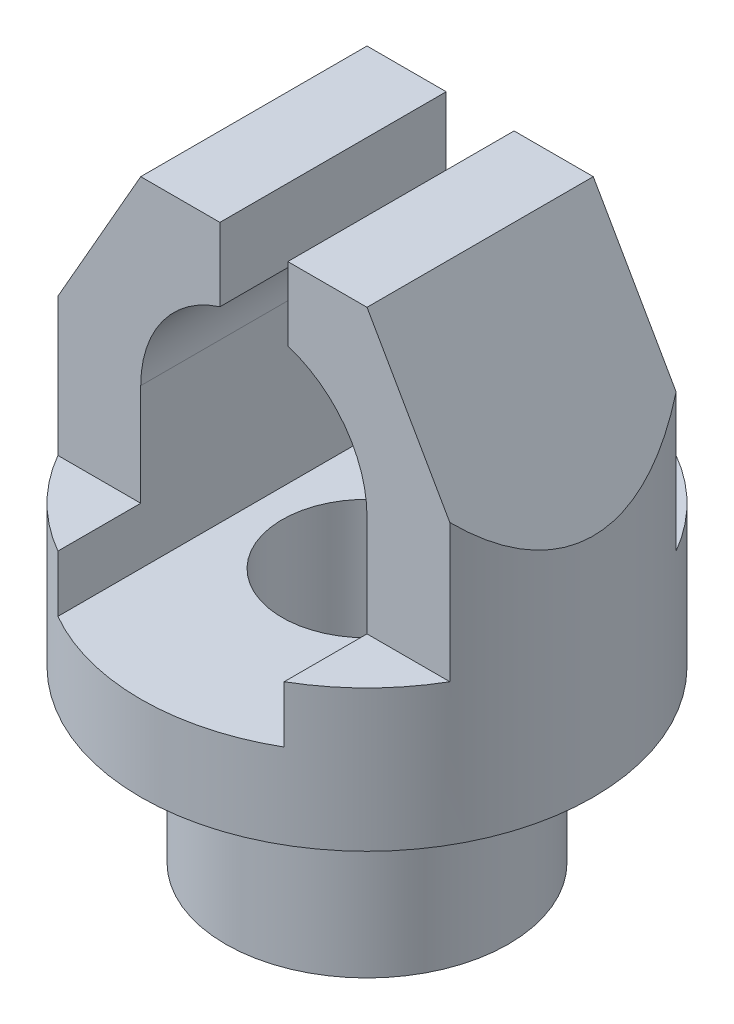
ISO-10303-21;
HEADER;
FILE_DESCRIPTION(('STEP AP214'),'2;1');
FILE_NAME('part.step','',(''),(''),'','','');
FILE_SCHEMA(('AUTOMOTIVE_DESIGN { 1 0 10303 214 1 1 1 1 }'));
ENDSEC;
DATA;
#1=APPLICATION_CONTEXT('core data for automotive mechanical design processes');
#2=APPLICATION_PROTOCOL_DEFINITION('international standard','automotive_design',2000,#1);
#3=PRODUCT_CONTEXT('',#1,'mechanical');
#4=PRODUCT('Part','Part','',(#3));
#5=PRODUCT_RELATED_PRODUCT_CATEGORY('part','',(#4));
#6=PRODUCT_DEFINITION_FORMATION('','',#4);
#7=PRODUCT_DEFINITION_CONTEXT('part definition',#1,'design');
#8=PRODUCT_DEFINITION('design','',#6,#7);
#9=PRODUCT_DEFINITION_SHAPE('','',#8);
#10=(LENGTH_UNIT() NAMED_UNIT(*) SI_UNIT(.MILLI.,.METRE.));
#11=(NAMED_UNIT(*) PLANE_ANGLE_UNIT() SI_UNIT($,.RADIAN.));
#12=(NAMED_UNIT(*) SI_UNIT($,.STERADIAN.) SOLID_ANGLE_UNIT());
#13=UNCERTAINTY_MEASURE_WITH_UNIT(LENGTH_MEASURE(1.E-05),#10,'distance_accuracy_value','');
#14=(GEOMETRIC_REPRESENTATION_CONTEXT(3) GLOBAL_UNCERTAINTY_ASSIGNED_CONTEXT((#13)) GLOBAL_UNIT_ASSIGNED_CONTEXT((#10,
#11,#12)) REPRESENTATION_CONTEXT('',''));
#15=CARTESIAN_POINT('',(0.,0.,0.));
#16=DIRECTION('',(0.,0.,1.));
#17=DIRECTION('',(1.,0.,0.));
#18=AXIS2_PLACEMENT_3D('',#15,#16,#17);
#19=CARTESIAN_POINT('',(40.,105.,0.));
#20=DIRECTION('',(0.,1.,0.));
#21=DIRECTION('',(0.,0.,1.));
#22=AXIS2_PLACEMENT_3D('',#19,#20,#21);
#23=PLANE('',#22);
#24=DIRECTION('',(0.,0.,1.));
#25=VECTOR('',#24,1.);
#26=CARTESIAN_POINT('',(-6.,105.,-40.));
#27=LINE('',#26,#25);
#28=CARTESIAN_POINT('',(-6.,105.,-20.));
#29=VERTEX_POINT('',#28);
#30=CARTESIAN_POINT('',(-6.,105.,20.));
#31=VERTEX_POINT('',#30);
#32=EDGE_CURVE('E335',#29,#31,#27,.T.);
#33=ORIENTED_EDGE('',*,*,#32,.F.);
#34=DIRECTION('',(1.,0.,0.));
#35=VECTOR('',#34,1.);
#36=CARTESIAN_POINT('',(40.,105.,-20.));
#37=LINE('',#36,#35);
#38=CARTESIAN_POINT('',(-20.,105.,-20.));
#39=VERTEX_POINT('',#38);
#40=EDGE_CURVE('E265',#39,#29,#37,.T.);
#41=ORIENTED_EDGE('',*,*,#40,.F.);
#42=DIRECTION('',(0.,0.,1.));
#43=VECTOR('',#42,1.);
#44=CARTESIAN_POINT('',(-20.,105.,-40.));
#45=LINE('',#44,#43);
#46=CARTESIAN_POINT('',(-20.,105.,20.));
#47=VERTEX_POINT('',#46);
#48=EDGE_CURVE('E321',#39,#47,#45,.T.);
#49=ORIENTED_EDGE('',*,*,#48,.T.);
#50=DIRECTION('',(-1.,0.,0.));
#51=VECTOR('',#50,1.);
#52=CARTESIAN_POINT('',(40.,105.,20.));
#53=LINE('',#52,#51);
#54=EDGE_CURVE('E263',#31,#47,#53,.T.);
#55=ORIENTED_EDGE('',*,*,#54,.F.);
#56=EDGE_LOOP('',(#33,#41,#49,#55));
#57=FACE_BOUND('',#56,.T.);
#58=ADVANCED_FACE('F39',(#57),#23,.T.);
#59=CARTESIAN_POINT('',(-40.,55.,-40.));
#60=DIRECTION('',(0.,-1.,0.));
#61=DIRECTION('',(0.,0.,-1.));
#62=AXIS2_PLACEMENT_3D('',#59,#60,#61);
#63=PLANE('',#62);
#64=DIRECTION('',(1.,0.,0.));
#65=VECTOR('',#64,1.);
#66=CARTESIAN_POINT('',(-40.,55.,-20.));
#67=LINE('',#66,#65);
#68=CARTESIAN_POINT('',(-34.6410161513775,55.,-20.));
#69=VERTEX_POINT('',#68);
#70=CARTESIAN_POINT('',(-20.,55.,-20.));
#71=VERTEX_POINT('',#70);
#72=EDGE_CURVE('E237',#69,#71,#67,.T.);
#73=ORIENTED_EDGE('',*,*,#72,.T.);
#74=DIRECTION('',(0.,0.,-1.));
#75=VECTOR('',#74,1.);
#76=CARTESIAN_POINT('',(-20.,55.,-40.));
#77=LINE('',#76,#75);
#78=CARTESIAN_POINT('',(-20.,55.,-34.6410161513775));
#79=VERTEX_POINT('',#78);
#80=EDGE_CURVE('E208',#71,#79,#77,.T.);
#81=ORIENTED_EDGE('',*,*,#80,.T.);
#82=CARTESIAN_POINT('',(0.,55.,0.));
#83=DIRECTION('',(0.,-1.,0.));
#84=DIRECTION('',(0.,0.,-1.));
#85=AXIS2_PLACEMENT_3D('',#82,#83,#84);
#86=CIRCLE('',#85,40.);
#87=EDGE_CURVE('E271',#79,#69,#86,.F.);
#88=ORIENTED_EDGE('',*,*,#87,.T.);
#89=EDGE_LOOP('',(#73,#81,#88));
#90=FACE_BOUND('',#89,.T.);
#91=ADVANCED_FACE('F360',(#90),#63,.F.);
#92=CARTESIAN_POINT('',(-40.,105.,-20.));
#93=DIRECTION('',(0.,0.,1.));
#94=DIRECTION('',(0.,-1.,0.));
#95=AXIS2_PLACEMENT_3D('',#92,#93,#94);
#96=PLANE('',#95);
#97=CARTESIAN_POINT('',(0.,73.,-20.));
#98=DIRECTION('',(0.,0.,1.));
#99=DIRECTION('',(0.,-1.,0.));
#100=AXIS2_PLACEMENT_3D('',#97,#98,#99);
#101=CIRCLE('',#100,20.);
#102=CARTESIAN_POINT('',(-6.,92.0787840283389,-20.));
#103=VERTEX_POINT('',#102);
#104=CARTESIAN_POINT('',(-20.,73.,-20.));
#105=VERTEX_POINT('',#104);
#106=EDGE_CURVE('E219',#103,#105,#101,.T.);
#107=ORIENTED_EDGE('',*,*,#106,.T.);
#108=DIRECTION('',(0.,-1.,0.));
#109=VECTOR('',#108,1.);
#110=CARTESIAN_POINT('',(-20.,105.,-20.));
#111=LINE('',#110,#109);
#112=EDGE_CURVE('E202',#105,#71,#111,.T.);
#113=ORIENTED_EDGE('',*,*,#112,.T.);
#114=ORIENTED_EDGE('',*,*,#72,.F.);
#115=DIRECTION('',(0.,-1.,0.));
#116=VECTOR('',#115,1.);
#117=CARTESIAN_POINT('',(-34.6410161513775,0.,-20.));
#118=LINE('',#117,#116);
#119=CARTESIAN_POINT('',(-34.6410161513775,79.3782217350893,-20.));
#120=VERTEX_POINT('',#119);
#121=EDGE_CURVE('E238',#69,#120,#118,.F.);
#122=ORIENTED_EDGE('',*,*,#121,.T.);
#123=DIRECTION('',(0.496138938356834,0.868243142124459,0.));
#124=VECTOR('',#123,1.);
#125=CARTESIAN_POINT('',(-24.9230769230769,96.3846153846154,-20.));
#126=LINE('',#125,#124);
#127=EDGE_CURVE('E171',#120,#39,#126,.T.);
#128=ORIENTED_EDGE('',*,*,#127,.T.);
#129=ORIENTED_EDGE('',*,*,#40,.T.);
#130=DIRECTION('',(0.,-1.,0.));
#131=VECTOR('',#130,1.);
#132=CARTESIAN_POINT('',(-6.,105.,-20.));
#133=LINE('',#132,#131);
#134=EDGE_CURVE('E220',#29,#103,#133,.T.);
#135=ORIENTED_EDGE('',*,*,#134,.T.);
#136=EDGE_LOOP('',(#107,#113,#114,#122,#128,#129,#135));
#137=FACE_BOUND('',#136,.T.);
#138=ADVANCED_FACE('F357',(#137),#96,.F.);
#139=CARTESIAN_POINT('',(-40.,105.,20.));
#140=DIRECTION('',(0.,0.,-1.));
#141=DIRECTION('',(0.,1.,0.));
#142=AXIS2_PLACEMENT_3D('',#139,#140,#141);
#143=PLANE('',#142);
#144=DIRECTION('',(1.,0.,0.));
#145=VECTOR('',#144,1.);
#146=CARTESIAN_POINT('',(-40.,55.,20.));
#147=LINE('',#146,#145);
#148=CARTESIAN_POINT('',(-34.6410161513775,55.,20.));
#149=VERTEX_POINT('',#148);
#150=CARTESIAN_POINT('',(-20.,55.,20.));
#151=VERTEX_POINT('',#150);
#152=EDGE_CURVE('E232',#149,#151,#147,.T.);
#153=ORIENTED_EDGE('',*,*,#152,.T.);
#154=DIRECTION('',(0.,1.,0.));
#155=VECTOR('',#154,1.);
#156=CARTESIAN_POINT('',(-20.,105.,20.));
#157=LINE('',#156,#155);
#158=CARTESIAN_POINT('',(-20.,73.,20.));
#159=VERTEX_POINT('',#158);
#160=EDGE_CURVE('E200',#151,#159,#157,.T.);
#161=ORIENTED_EDGE('',*,*,#160,.T.);
#162=CARTESIAN_POINT('',(0.,73.,20.));
#163=DIRECTION('',(0.,0.,-1.));
#164=DIRECTION('',(0.,1.,0.));
#165=AXIS2_PLACEMENT_3D('',#162,#163,#164);
#166=CIRCLE('',#165,20.);
#167=CARTESIAN_POINT('',(-6.,92.0787840283389,20.));
#168=VERTEX_POINT('',#167);
#169=EDGE_CURVE('E292',#159,#168,#166,.T.);
#170=ORIENTED_EDGE('',*,*,#169,.T.);
#171=DIRECTION('',(0.,1.,0.));
#172=VECTOR('',#171,1.);
#173=CARTESIAN_POINT('',(-6.,105.,20.));
#174=LINE('',#173,#172);
#175=EDGE_CURVE('E290',#168,#31,#174,.T.);
#176=ORIENTED_EDGE('',*,*,#175,.T.);
#177=ORIENTED_EDGE('',*,*,#54,.T.);
#178=DIRECTION('',(-0.496138938356834,-0.868243142124459,0.));
#179=VECTOR('',#178,1.);
#180=CARTESIAN_POINT('',(-24.9230769230769,96.3846153846154,20.));
#181=LINE('',#180,#179);
#182=CARTESIAN_POINT('',(-34.6410161513776,79.3782217350892,20.));
#183=VERTEX_POINT('',#182);
#184=EDGE_CURVE('E283',#47,#183,#181,.T.);
#185=ORIENTED_EDGE('',*,*,#184,.T.);
#186=DIRECTION('',(0.,-1.,0.));
#187=VECTOR('',#186,1.);
#188=CARTESIAN_POINT('',(-34.6410161513775,0.,20.));
#189=LINE('',#188,#187);
#190=EDGE_CURVE('E242',#183,#149,#189,.T.);
#191=ORIENTED_EDGE('',*,*,#190,.T.);
#192=EDGE_LOOP('',(#153,#161,#170,#176,#177,#185,#191));
#193=FACE_BOUND('',#192,.T.);
#194=ADVANCED_FACE('F345',(#193),#143,.F.);
#195=CARTESIAN_POINT('',(-40.,55.,40.));
#196=DIRECTION('',(0.,-1.,0.));
#197=DIRECTION('',(0.,0.,-1.));
#198=AXIS2_PLACEMENT_3D('',#195,#196,#197);
#199=PLANE('',#198);
#200=CARTESIAN_POINT('',(0.,55.,0.));
#201=DIRECTION('',(0.,-1.,0.));
#202=DIRECTION('',(0.,0.,-1.));
#203=AXIS2_PLACEMENT_3D('',#200,#201,#202);
#204=CIRCLE('',#203,40.);
#205=CARTESIAN_POINT('',(-20.,55.,34.6410161513775));
#206=VERTEX_POINT('',#205);
#207=EDGE_CURVE('E275',#149,#206,#204,.F.);
#208=ORIENTED_EDGE('',*,*,#207,.T.);
#209=DIRECTION('',(0.,0.,-1.));
#210=VECTOR('',#209,1.);
#211=CARTESIAN_POINT('',(-20.,55.,40.));
#212=LINE('',#211,#210);
#213=EDGE_CURVE('E279',#206,#151,#212,.T.);
#214=ORIENTED_EDGE('',*,*,#213,.T.);
#215=ORIENTED_EDGE('',*,*,#152,.F.);
#216=EDGE_LOOP('',(#208,#214,#215));
#217=FACE_BOUND('',#216,.T.);
#218=ADVANCED_FACE('F346',(#217),#199,.F.);
#219=CARTESIAN_POINT('',(0.,0.,0.));
#220=DIRECTION('',(0.,-1.,0.));
#221=DIRECTION('',(0.,0.,-1.));
#222=AXIS2_PLACEMENT_3D('',#219,#220,#221);
#223=CYLINDRICAL_SURFACE('',#222,15.);
#224=CARTESIAN_POINT('',(0.,45.,0.));
#225=DIRECTION('',(0.,-1.,0.));
#226=DIRECTION('',(0.,0.,-1.));
#227=AXIS2_PLACEMENT_3D('',#224,#225,#226);
#228=CIRCLE('',#227,15.);
#229=CARTESIAN_POINT('',(0.,45.,-15.));
#230=VERTEX_POINT('',#229);
#231=EDGE_CURVE('E227',#230,#230,#228,.T.);
#232=ORIENTED_EDGE('',*,*,#231,.F.);
#233=EDGE_LOOP('',(#232));
#234=FACE_BOUND('',#233,.T.);
#235=CARTESIAN_POINT('',(0.,0.,0.));
#236=DIRECTION('',(0.,-1.,0.));
#237=DIRECTION('',(0.,0.,-1.));
#238=AXIS2_PLACEMENT_3D('',#235,#236,#237);
#239=CIRCLE('',#238,15.);
#240=CARTESIAN_POINT('',(0.,0.,-15.));
#241=VERTEX_POINT('',#240);
#242=EDGE_CURVE('E260',#241,#241,#239,.T.);
#243=ORIENTED_EDGE('',*,*,#242,.T.);
#244=EDGE_LOOP('',(#243));
#245=FACE_BOUND('',#244,.T.);
#246=ADVANCED_FACE('F41',(#234,#245),#223,.F.);
#247=CARTESIAN_POINT('',(15.,0.,0.));
#248=DIRECTION('',(0.,-1.,0.));
#249=DIRECTION('',(0.,0.,-1.));
#250=AXIS2_PLACEMENT_3D('',#247,#248,#249);
#251=PLANE('',#250);
#252=CARTESIAN_POINT('',(0.,0.,0.));
#253=DIRECTION('',(0.,-1.,0.));
#254=DIRECTION('',(0.,0.,-1.));
#255=AXIS2_PLACEMENT_3D('',#252,#253,#254);
#256=CIRCLE('',#255,25.);
#257=CARTESIAN_POINT('',(0.,0.,-25.));
#258=VERTEX_POINT('',#257);
#259=EDGE_CURVE('E255',#258,#258,#256,.T.);
#260=ORIENTED_EDGE('',*,*,#259,.T.);
#261=EDGE_LOOP('',(#260));
#262=FACE_BOUND('',#261,.T.);
#263=ORIENTED_EDGE('',*,*,#242,.F.);
#264=EDGE_LOOP('',(#263));
#265=FACE_BOUND('',#264,.T.);
#266=ADVANCED_FACE('F394',(#262,#265),#251,.T.);
#267=CARTESIAN_POINT('',(0.,0.,0.));
#268=DIRECTION('',(0.,-1.,0.));
#269=DIRECTION('',(0.,0.,-1.));
#270=AXIS2_PLACEMENT_3D('',#267,#268,#269);
#271=CYLINDRICAL_SURFACE('',#270,25.);
#272=CARTESIAN_POINT('',(0.,30.,0.));
#273=DIRECTION('',(0.,-1.,0.));
#274=DIRECTION('',(0.,0.,-1.));
#275=AXIS2_PLACEMENT_3D('',#272,#273,#274);
#276=CIRCLE('',#275,25.);
#277=CARTESIAN_POINT('',(0.,30.,-25.));
#278=VERTEX_POINT('',#277);
#279=EDGE_CURVE('E253',#278,#278,#276,.T.);
#280=ORIENTED_EDGE('',*,*,#279,.T.);
#281=EDGE_LOOP('',(#280));
#282=FACE_BOUND('',#281,.T.);
#283=ORIENTED_EDGE('',*,*,#259,.F.);
#284=EDGE_LOOP('',(#283));
#285=FACE_BOUND('',#284,.T.);
#286=ADVANCED_FACE('F386',(#282,#285),#271,.T.);
#287=CARTESIAN_POINT('',(25.,30.,0.));
#288=DIRECTION('',(0.,-1.,0.));
#289=DIRECTION('',(0.,0.,-1.));
#290=AXIS2_PLACEMENT_3D('',#287,#288,#289);
#291=PLANE('',#290);
#292=CARTESIAN_POINT('',(0.,30.,0.));
#293=DIRECTION('',(0.,-1.,0.));
#294=DIRECTION('',(0.,0.,-1.));
#295=AXIS2_PLACEMENT_3D('',#292,#293,#294);
#296=CIRCLE('',#295,40.);
#297=CARTESIAN_POINT('',(0.,30.,-40.));
#298=VERTEX_POINT('',#297);
#299=EDGE_CURVE('E250',#298,#298,#296,.T.);
#300=ORIENTED_EDGE('',*,*,#299,.T.);
#301=EDGE_LOOP('',(#300));
#302=FACE_BOUND('',#301,.T.);
#303=ORIENTED_EDGE('',*,*,#279,.F.);
#304=EDGE_LOOP('',(#303));
#305=FACE_BOUND('',#304,.T.);
#306=ADVANCED_FACE('F390',(#302,#305),#291,.T.);
#307=CARTESIAN_POINT('',(0.,0.,0.));
#308=DIRECTION('',(0.,-1.,0.));
#309=DIRECTION('',(0.,0.,-1.));
#310=AXIS2_PLACEMENT_3D('',#307,#308,#309);
#311=CYLINDRICAL_SURFACE('',#310,40.);
#312=DIRECTION('',(0.,-1.,0.));
#313=VECTOR('',#312,1.);
#314=CARTESIAN_POINT('',(34.6410161513775,0.,-20.));
#315=LINE('',#314,#313);
#316=CARTESIAN_POINT('',(34.6410161513775,79.3782217350893,-20.));
#317=VERTEX_POINT('',#316);
#318=CARTESIAN_POINT('',(34.6410161513775,55.,-20.));
#319=VERTEX_POINT('',#318);
#320=EDGE_CURVE('E231',#317,#319,#315,.T.);
#321=ORIENTED_EDGE('',*,*,#320,.F.);
#322=CARTESIAN_POINT('',(0.,140.,0.));
#323=DIRECTION('',(-0.868243142124459,-0.496138938356834,0.));
#324=DIRECTION('',(0.496138938356834,-0.868243142124459,0.));
#325=AXIS2_PLACEMENT_3D('',#322,#323,#324);
#326=ELLIPSE('',#325,80.6225774829855,40.);
#327=CARTESIAN_POINT('',(34.6410161513776,79.3782217350893,20.));
#328=VERTEX_POINT('',#327);
#329=EDGE_CURVE('E224',#328,#317,#326,.F.);
#330=ORIENTED_EDGE('',*,*,#329,.F.);
#331=DIRECTION('',(0.,-1.,0.));
#332=VECTOR('',#331,1.);
#333=CARTESIAN_POINT('',(34.6410161513775,0.,20.));
#334=LINE('',#333,#332);
#335=CARTESIAN_POINT('',(34.6410161513775,55.,20.));
#336=VERTEX_POINT('',#335);
#337=EDGE_CURVE('E241',#336,#328,#334,.F.);
#338=ORIENTED_EDGE('',*,*,#337,.F.);
#339=CARTESIAN_POINT('',(20.,55.,34.6410161513775));
#340=VERTEX_POINT('',#339);
#341=EDGE_CURVE('E269',#340,#336,#204,.F.);
#342=ORIENTED_EDGE('',*,*,#341,.F.);
#343=DIRECTION('',(0.,-1.,0.));
#344=VECTOR('',#343,1.);
#345=CARTESIAN_POINT('',(20.,0.,34.6410161513775));
#346=LINE('',#345,#344);
#347=CARTESIAN_POINT('',(20.,45.,34.6410161513775));
#348=VERTEX_POINT('',#347);
#349=EDGE_CURVE('E192',#348,#340,#346,.F.);
#350=ORIENTED_EDGE('',*,*,#349,.F.);
#351=CARTESIAN_POINT('',(0.,45.,0.));
#352=DIRECTION('',(0.,-1.,0.));
#353=DIRECTION('',(0.,0.,-1.));
#354=AXIS2_PLACEMENT_3D('',#351,#352,#353);
#355=CIRCLE('',#354,40.);
#356=CARTESIAN_POINT('',(-20.,45.,34.6410161513775));
#357=VERTEX_POINT('',#356);
#358=EDGE_CURVE('E43',#357,#348,#355,.F.);
#359=ORIENTED_EDGE('',*,*,#358,.F.);
#360=DIRECTION('',(0.,-1.,0.));
#361=VECTOR('',#360,1.);
#362=CARTESIAN_POINT('',(-20.,0.,34.6410161513775));
#363=LINE('',#362,#361);
#364=EDGE_CURVE('E205',#206,#357,#363,.T.);
#365=ORIENTED_EDGE('',*,*,#364,.F.);
#366=ORIENTED_EDGE('',*,*,#207,.F.);
#367=ORIENTED_EDGE('',*,*,#190,.F.);
#368=CARTESIAN_POINT('',(0.,140.,0.));
#369=DIRECTION('',(0.868243142124459,-0.496138938356834,0.));
#370=DIRECTION('',(-0.496138938356834,-0.868243142124459,0.));
#371=AXIS2_PLACEMENT_3D('',#368,#369,#370);
#372=ELLIPSE('',#371,80.6225774829855,40.);
#373=EDGE_CURVE('E53',#120,#183,#372,.F.);
#374=ORIENTED_EDGE('',*,*,#373,.F.);
#375=ORIENTED_EDGE('',*,*,#121,.F.);
#376=ORIENTED_EDGE('',*,*,#87,.F.);
#377=DIRECTION('',(0.,-1.,0.));
#378=VECTOR('',#377,1.);
#379=CARTESIAN_POINT('',(-20.,0.,-34.6410161513775));
#380=LINE('',#379,#378);
#381=CARTESIAN_POINT('',(-20.,45.,-34.6410161513775));
#382=VERTEX_POINT('',#381);
#383=EDGE_CURVE('E211',#382,#79,#380,.F.);
#384=ORIENTED_EDGE('',*,*,#383,.F.);
#385=CARTESIAN_POINT('',(20.,45.,-34.6410161513775));
#386=VERTEX_POINT('',#385);
#387=EDGE_CURVE('E11',#386,#382,#355,.F.);
#388=ORIENTED_EDGE('',*,*,#387,.F.);
#389=DIRECTION('',(0.,-1.,0.));
#390=VECTOR('',#389,1.);
#391=CARTESIAN_POINT('',(20.,0.,-34.6410161513775));
#392=LINE('',#391,#390);
#393=CARTESIAN_POINT('',(20.,55.,-34.6410161513775));
#394=VERTEX_POINT('',#393);
#395=EDGE_CURVE('E195',#394,#386,#392,.T.);
#396=ORIENTED_EDGE('',*,*,#395,.F.);
#397=EDGE_CURVE('E270',#319,#394,#86,.F.);
#398=ORIENTED_EDGE('',*,*,#397,.F.);
#399=EDGE_LOOP('',(#321,#330,#338,#342,#350,#359,#365,#366,#367,#374,#375,#376,#384,#388,#396,#398));
#400=FACE_BOUND('',#399,.T.);
#401=ORIENTED_EDGE('',*,*,#299,.F.);
#402=EDGE_LOOP('',(#401));
#403=FACE_BOUND('',#402,.T.);
#404=ADVANCED_FACE('F315',(#400,#403),#311,.T.);
#405=DIRECTION('',(0.,0.,1.));
#406=VECTOR('',#405,1.);
#407=CARTESIAN_POINT('',(20.,105.,-40.));
#408=LINE('',#407,#406);
#409=CARTESIAN_POINT('',(20.,105.,-20.));
#410=VERTEX_POINT('',#409);
#411=CARTESIAN_POINT('',(20.,105.,20.));
#412=VERTEX_POINT('',#411);
#413=EDGE_CURVE('E64',#410,#412,#408,.T.);
#414=ORIENTED_EDGE('',*,*,#413,.F.);
#415=CARTESIAN_POINT('',(6.,105.,-20.));
#416=VERTEX_POINT('',#415);
#417=EDGE_CURVE('E257',#416,#410,#37,.T.);
#418=ORIENTED_EDGE('',*,*,#417,.F.);
#419=DIRECTION('',(0.,0.,1.));
#420=VECTOR('',#419,1.);
#421=CARTESIAN_POINT('',(6.,105.,-40.));
#422=LINE('',#421,#420);
#423=CARTESIAN_POINT('',(6.,105.,20.));
#424=VERTEX_POINT('',#423);
#425=EDGE_CURVE('E328',#416,#424,#422,.T.);
#426=ORIENTED_EDGE('',*,*,#425,.T.);
#427=EDGE_CURVE('E266',#412,#424,#53,.T.);
#428=ORIENTED_EDGE('',*,*,#427,.F.);
#429=EDGE_LOOP('',(#414,#418,#426,#428));
#430=FACE_BOUND('',#429,.T.);
#431=ADVANCED_FACE('F363',(#430),#23,.T.);
#432=ORIENTED_EDGE('',*,*,#397,.T.);
#433=DIRECTION('',(0.,0.,1.));
#434=VECTOR('',#433,1.);
#435=CARTESIAN_POINT('',(20.,55.,-40.));
#436=LINE('',#435,#434);
#437=CARTESIAN_POINT('',(20.,55.,-20.));
#438=VERTEX_POINT('',#437);
#439=EDGE_CURVE('E186',#394,#438,#436,.T.);
#440=ORIENTED_EDGE('',*,*,#439,.T.);
#441=EDGE_CURVE('E190',#438,#319,#67,.T.);
#442=ORIENTED_EDGE('',*,*,#441,.T.);
#443=EDGE_LOOP('',(#432,#440,#442));
#444=FACE_BOUND('',#443,.T.);
#445=ADVANCED_FACE('F370',(#444),#63,.F.);
#446=ORIENTED_EDGE('',*,*,#417,.T.);
#447=DIRECTION('',(0.496138938356834,-0.868243142124459,0.));
#448=VECTOR('',#447,1.);
#449=CARTESIAN_POINT('',(5.23076923076925,130.846153846154,-20.));
#450=LINE('',#449,#448);
#451=EDGE_CURVE('E223',#410,#317,#450,.T.);
#452=ORIENTED_EDGE('',*,*,#451,.T.);
#453=ORIENTED_EDGE('',*,*,#320,.T.);
#454=ORIENTED_EDGE('',*,*,#441,.F.);
#455=DIRECTION('',(0.,1.,0.));
#456=VECTOR('',#455,1.);
#457=CARTESIAN_POINT('',(20.,105.,-20.));
#458=LINE('',#457,#456);
#459=CARTESIAN_POINT('',(20.,73.,-20.));
#460=VERTEX_POINT('',#459);
#461=EDGE_CURVE('E176',#438,#460,#458,.T.);
#462=ORIENTED_EDGE('',*,*,#461,.T.);
#463=CARTESIAN_POINT('',(0.,73.,-20.));
#464=DIRECTION('',(0.,0.,1.));
#465=DIRECTION('',(0.,-1.,0.));
#466=AXIS2_PLACEMENT_3D('',#463,#464,#465);
#467=CIRCLE('',#466,20.);
#468=CARTESIAN_POINT('',(6.,92.0787840283389,-20.));
#469=VERTEX_POINT('',#468);
#470=EDGE_CURVE('E163',#460,#469,#467,.T.);
#471=ORIENTED_EDGE('',*,*,#470,.T.);
#472=DIRECTION('',(0.,1.,0.));
#473=VECTOR('',#472,1.);
#474=CARTESIAN_POINT('',(6.,105.,-20.));
#475=LINE('',#474,#473);
#476=EDGE_CURVE('E175',#469,#416,#475,.T.);
#477=ORIENTED_EDGE('',*,*,#476,.T.);
#478=EDGE_LOOP('',(#446,#452,#453,#454,#462,#471,#477));
#479=FACE_BOUND('',#478,.T.);
#480=ADVANCED_FACE('F189',(#479),#96,.F.);
#481=ORIENTED_EDGE('',*,*,#337,.T.);
#482=DIRECTION('',(-0.496138938356834,0.868243142124459,0.));
#483=VECTOR('',#482,1.);
#484=CARTESIAN_POINT('',(5.23076923076925,130.846153846154,20.));
#485=LINE('',#484,#483);
#486=EDGE_CURVE('E291',#328,#412,#485,.T.);
#487=ORIENTED_EDGE('',*,*,#486,.T.);
#488=ORIENTED_EDGE('',*,*,#427,.T.);
#489=DIRECTION('',(0.,-1.,0.));
#490=VECTOR('',#489,1.);
#491=CARTESIAN_POINT('',(6.,105.,20.));
#492=LINE('',#491,#490);
#493=CARTESIAN_POINT('',(6.,92.0787840283389,20.));
#494=VERTEX_POINT('',#493);
#495=EDGE_CURVE('E281',#424,#494,#492,.T.);
#496=ORIENTED_EDGE('',*,*,#495,.T.);
#497=CARTESIAN_POINT('',(0.,73.,20.));
#498=DIRECTION('',(0.,0.,-1.));
#499=DIRECTION('',(0.,1.,0.));
#500=AXIS2_PLACEMENT_3D('',#497,#498,#499);
#501=CIRCLE('',#500,20.);
#502=CARTESIAN_POINT('',(20.,73.,20.));
#503=VERTEX_POINT('',#502);
#504=EDGE_CURVE('E282',#494,#503,#501,.T.);
#505=ORIENTED_EDGE('',*,*,#504,.T.);
#506=DIRECTION('',(0.,-1.,0.));
#507=VECTOR('',#506,1.);
#508=CARTESIAN_POINT('',(20.,105.,20.));
#509=LINE('',#508,#507);
#510=CARTESIAN_POINT('',(20.,55.,20.));
#511=VERTEX_POINT('',#510);
#512=EDGE_CURVE('E185',#503,#511,#509,.T.);
#513=ORIENTED_EDGE('',*,*,#512,.T.);
#514=EDGE_CURVE('E233',#511,#336,#147,.T.);
#515=ORIENTED_EDGE('',*,*,#514,.T.);
#516=EDGE_LOOP('',(#481,#487,#488,#496,#505,#513,#515));
#517=FACE_BOUND('',#516,.T.);
#518=ADVANCED_FACE('F319',(#517),#143,.F.);
#519=ORIENTED_EDGE('',*,*,#514,.F.);
#520=DIRECTION('',(0.,0.,1.));
#521=VECTOR('',#520,1.);
#522=CARTESIAN_POINT('',(20.,55.,40.));
#523=LINE('',#522,#521);
#524=EDGE_CURVE('E274',#511,#340,#523,.T.);
#525=ORIENTED_EDGE('',*,*,#524,.T.);
#526=ORIENTED_EDGE('',*,*,#341,.T.);
#527=EDGE_LOOP('',(#519,#525,#526));
#528=FACE_BOUND('',#527,.T.);
#529=ADVANCED_FACE('F317',(#528),#199,.F.);
#530=CARTESIAN_POINT('',(0.,73.,-40.));
#531=DIRECTION('',(0.,0.,1.));
#532=DIRECTION('',(1.,0.,0.));
#533=AXIS2_PLACEMENT_3D('',#530,#531,#532);
#534=CYLINDRICAL_SURFACE('',#533,20.);
#535=DIRECTION('',(0.,0.,1.));
#536=VECTOR('',#535,1.);
#537=CARTESIAN_POINT('',(-6.,92.0787840283389,-40.));
#538=LINE('',#537,#536);
#539=EDGE_CURVE('E331',#103,#168,#538,.T.);
#540=ORIENTED_EDGE('',*,*,#539,.T.);
#541=ORIENTED_EDGE('',*,*,#169,.F.);
#542=DIRECTION('',(0.,0.,1.));
#543=VECTOR('',#542,1.);
#544=CARTESIAN_POINT('',(-20.,73.,-40.));
#545=LINE('',#544,#543);
#546=EDGE_CURVE('E326',#105,#159,#545,.T.);
#547=ORIENTED_EDGE('',*,*,#546,.F.);
#548=ORIENTED_EDGE('',*,*,#106,.F.);
#549=EDGE_LOOP('',(#540,#541,#547,#548));
#550=FACE_BOUND('',#549,.T.);
#551=ADVANCED_FACE('F430',(#550),#534,.F.);
#552=CARTESIAN_POINT('',(-6.,105.,-40.));
#553=DIRECTION('',(-1.,0.,0.));
#554=DIRECTION('',(0.,-1.,0.));
#555=AXIS2_PLACEMENT_3D('',#552,#553,#554);
#556=PLANE('',#555);
#557=ORIENTED_EDGE('',*,*,#32,.T.);
#558=ORIENTED_EDGE('',*,*,#175,.F.);
#559=ORIENTED_EDGE('',*,*,#539,.F.);
#560=ORIENTED_EDGE('',*,*,#134,.F.);
#561=EDGE_LOOP('',(#557,#558,#559,#560));
#562=FACE_BOUND('',#561,.T.);
#563=ADVANCED_FACE('F431',(#562),#556,.F.);
#564=CARTESIAN_POINT('',(6.,105.,-40.));
#565=DIRECTION('',(1.,0.,0.));
#566=DIRECTION('',(0.,1.,0.));
#567=AXIS2_PLACEMENT_3D('',#564,#565,#566);
#568=PLANE('',#567);
#569=DIRECTION('',(0.,0.,1.));
#570=VECTOR('',#569,1.);
#571=CARTESIAN_POINT('',(6.,92.0787840283389,-40.));
#572=LINE('',#571,#570);
#573=EDGE_CURVE('E168',#469,#494,#572,.T.);
#574=ORIENTED_EDGE('',*,*,#573,.T.);
#575=ORIENTED_EDGE('',*,*,#495,.F.);
#576=ORIENTED_EDGE('',*,*,#425,.F.);
#577=ORIENTED_EDGE('',*,*,#476,.F.);
#578=EDGE_LOOP('',(#574,#575,#576,#577));
#579=FACE_BOUND('',#578,.T.);
#580=ADVANCED_FACE('F365',(#579),#568,.F.);
#581=CARTESIAN_POINT('',(0.,73.,-40.));
#582=DIRECTION('',(0.,0.,1.));
#583=DIRECTION('',(1.,0.,0.));
#584=AXIS2_PLACEMENT_3D('',#581,#582,#583);
#585=CYLINDRICAL_SURFACE('',#584,20.);
#586=DIRECTION('',(0.,0.,1.));
#587=VECTOR('',#586,1.);
#588=CARTESIAN_POINT('',(20.,73.,-40.));
#589=LINE('',#588,#587);
#590=EDGE_CURVE('E170',#460,#503,#589,.T.);
#591=ORIENTED_EDGE('',*,*,#590,.T.);
#592=ORIENTED_EDGE('',*,*,#504,.F.);
#593=ORIENTED_EDGE('',*,*,#573,.F.);
#594=ORIENTED_EDGE('',*,*,#470,.F.);
#595=EDGE_LOOP('',(#591,#592,#593,#594));
#596=FACE_BOUND('',#595,.T.);
#597=ADVANCED_FACE('F167',(#596),#585,.F.);
#598=CARTESIAN_POINT('',(-20.,45.,-40.));
#599=DIRECTION('',(-1.,0.,0.));
#600=DIRECTION('',(0.,0.,1.));
#601=AXIS2_PLACEMENT_3D('',#598,#599,#600);
#602=PLANE('',#601);
#603=ORIENTED_EDGE('',*,*,#383,.T.);
#604=ORIENTED_EDGE('',*,*,#80,.F.);
#605=ORIENTED_EDGE('',*,*,#112,.F.);
#606=ORIENTED_EDGE('',*,*,#546,.T.);
#607=ORIENTED_EDGE('',*,*,#160,.F.);
#608=ORIENTED_EDGE('',*,*,#213,.F.);
#609=ORIENTED_EDGE('',*,*,#364,.T.);
#610=DIRECTION('',(0.,0.,1.));
#611=VECTOR('',#610,1.);
#612=CARTESIAN_POINT('',(-20.,45.,-40.));
#613=LINE('',#612,#611);
#614=EDGE_CURVE('E301',#382,#357,#613,.T.);
#615=ORIENTED_EDGE('',*,*,#614,.F.);
#616=EDGE_LOOP('',(#603,#604,#605,#606,#607,#608,#609,#615));
#617=FACE_BOUND('',#616,.T.);
#618=ADVANCED_FACE('F336',(#617),#602,.F.);
#619=CARTESIAN_POINT('',(20.,45.,-40.));
#620=DIRECTION('',(1.,0.,0.));
#621=DIRECTION('',(0.,0.,-1.));
#622=AXIS2_PLACEMENT_3D('',#619,#620,#621);
#623=PLANE('',#622);
#624=ORIENTED_EDGE('',*,*,#395,.T.);
#625=DIRECTION('',(0.,0.,1.));
#626=VECTOR('',#625,1.);
#627=CARTESIAN_POINT('',(20.,45.,-40.));
#628=LINE('',#627,#626);
#629=EDGE_CURVE('E181',#386,#348,#628,.T.);
#630=ORIENTED_EDGE('',*,*,#629,.T.);
#631=ORIENTED_EDGE('',*,*,#349,.T.);
#632=ORIENTED_EDGE('',*,*,#524,.F.);
#633=ORIENTED_EDGE('',*,*,#512,.F.);
#634=ORIENTED_EDGE('',*,*,#590,.F.);
#635=ORIENTED_EDGE('',*,*,#461,.F.);
#636=ORIENTED_EDGE('',*,*,#439,.F.);
#637=EDGE_LOOP('',(#624,#630,#631,#632,#633,#634,#635,#636));
#638=FACE_BOUND('',#637,.T.);
#639=ADVANCED_FACE('F180',(#638),#623,.F.);
#640=CARTESIAN_POINT('',(-20.,45.,-40.));
#641=DIRECTION('',(0.,-1.,0.));
#642=DIRECTION('',(0.,0.,-1.));
#643=AXIS2_PLACEMENT_3D('',#640,#641,#642);
#644=PLANE('',#643);
#645=ORIENTED_EDGE('',*,*,#231,.T.);
#646=EDGE_LOOP('',(#645));
#647=FACE_BOUND('',#646,.T.);
#648=ORIENTED_EDGE('',*,*,#614,.T.);
#649=ORIENTED_EDGE('',*,*,#358,.T.);
#650=ORIENTED_EDGE('',*,*,#629,.F.);
#651=ORIENTED_EDGE('',*,*,#387,.T.);
#652=EDGE_LOOP('',(#648,#649,#650,#651));
#653=FACE_BOUND('',#652,.T.);
#654=ADVANCED_FACE('F302',(#647,#653),#644,.F.);
#655=CARTESIAN_POINT('',(-20.,105.,-40.));
#656=DIRECTION('',(0.868243142124459,-0.496138938356834,0.));
#657=DIRECTION('',(0.496138938356834,0.868243142124459,0.));
#658=AXIS2_PLACEMENT_3D('',#655,#656,#657);
#659=PLANE('',#658);
#660=ORIENTED_EDGE('',*,*,#127,.F.);
#661=ORIENTED_EDGE('',*,*,#373,.T.);
#662=ORIENTED_EDGE('',*,*,#184,.F.);
#663=ORIENTED_EDGE('',*,*,#48,.F.);
#664=EDGE_LOOP('',(#660,#661,#662,#663));
#665=FACE_BOUND('',#664,.T.);
#666=ADVANCED_FACE('F353',(#665),#659,.F.);
#667=CARTESIAN_POINT('',(20.,105.,-40.));
#668=DIRECTION('',(-0.868243142124459,-0.496138938356834,0.));
#669=DIRECTION('',(0.496138938356834,-0.868243142124459,0.));
#670=AXIS2_PLACEMENT_3D('',#667,#668,#669);
#671=PLANE('',#670);
#672=ORIENTED_EDGE('',*,*,#413,.T.);
#673=ORIENTED_EDGE('',*,*,#486,.F.);
#674=ORIENTED_EDGE('',*,*,#329,.T.);
#675=ORIENTED_EDGE('',*,*,#451,.F.);
#676=EDGE_LOOP('',(#672,#673,#674,#675));
#677=FACE_BOUND('',#676,.T.);
#678=ADVANCED_FACE('F418',(#677),#671,.F.);
#679=CLOSED_SHELL('',(#58,#91,#138,#194,#218,#246,#266,#286,#306,#404,#431,#445,#480,#518,#529,
#551,#563,#580,#597,#618,#639,#654,#666,#678));
#680=MANIFOLD_SOLID_BREP('B2',#679);
#681=ADVANCED_BREP_SHAPE_REPRESENTATION('',(#18,#680),#14);
#682=SHAPE_DEFINITION_REPRESENTATION(#9,#681);
ENDSEC;
END-ISO-10303-21;
